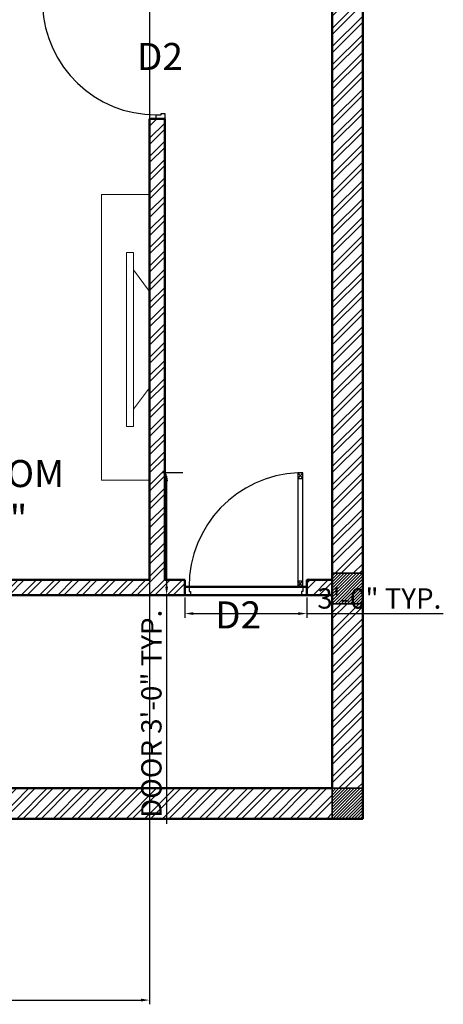
# Model space of a CAD drawing. Units: millimetres. Extents: x 20768 to 23556, y 50760 to 52704.
# Tile 13 of 36: x 21032 to 21157, y 51775 to 52066. Entities that reach past the tile are written whole.
import ezdxf

# ---------------------------------------------------------------- set-up
doc = ezdxf.new("R2010")
doc.units = ezdxf.units.MM
for name, color, linetype, lineweight in [('A-AREA-IDEN', 40, 'Continuous', 18), ('A-DOOR', 3, 'Continuous', 25), ('A-FURN', 8, 'Continuous', 18), ('A-WALL', 7, 'Continuous', 50), ('A-WALL-PATT', 8, 'Continuous', 13), ('S-ANNO-DIMS', 2, 'Continuous', 18), ('S-COLS', 20, 'Continuous', 35)]:
    doc.layers.add(name, color=color, linetype=linetype, lineweight=lineweight)
doc.styles.get("Standard").update_dxf_attribs({"font": 'arial.ttf'})
doc.dimstyles.new('ISO-25', dxfattribs={"dimtxt": 6, "dimasz": 2.5, "dimexe": 1.25, "dimexo": 0.625, "dimtad": 1, "dimdec": 0, "dimlunit": 3, "dimtxsty": 'Standard', "dimcen": 2.5, "dimadec": 0, "dimazin": 0, "dimtfac": 1, "dimtdec": 0, "dimtmove": 0, "dimatfit": 3, "dimfxl": 1, "dimarcsym": 0})
pattern_1 = [(45, (-81.1113, 0), (-2.69407684, 2.69407684), []), (45, (-79.3152, 0), (-2.69407684, 2.69407684), [])]
pattern_2 = [(45, (-81.11126, 0), (-0.449012806, 0.449012806), [])]

# ---------------------------------------------------------------- blocks, each defined once
blk = doc.blocks.new('Puerta 01')
for p, q in [((-0.7745, -0.0264), (-0.7368, -0.0584)), ((-0.7745, -0.0584), (-0.7368, -0.0264)), ((-0.7368, -0.0584), (-0.7368, -0.0264)), ((-0.028, -0.0584), (-0.0657, -0.0264)), ((-0.028, -0.0264), (-0.0657, -0.0584)), ((-0.0657, -0.0584), (-0.0657, -0.0264))]:
    blk.add_line(p, q)
for points in [[(-0.028, 0), (-0.028, -0.0264), (0.004, -0.0264), (0.004, -0.036), (0.028, -0.036), (0.028, 0)], [(-0.028, -0.0264), (-0.7745, -0.0264), (-0.7745, -0.0584), (-0.028, -0.0584)], [(0.004, -0.7736), (0.004, -0.764), (0.028, -0.764), (0.028, -0.8), (-0.028, -0.8), (-0.028, -0.7736)]]:
    blk.add_lwpolyline(points, close=True)
blk.add_arc((-0.028, -0.0264), 0.7472, 182.45453, 270)
blk = doc.blocks.new('tv')
for p, q in [((20989.25, 52437.95), (20993.93, 52444.3)), ((20989.25, 52409.51), (20993.93, 52403.15))]:
    blk.add_line(p, q)
for points in [[(20989.25, 52466.51), (21003.46, 52466.51), (21003.46, 52382.21), (20989.25, 52382.21)], [(20993.93, 52449.42), (20996.05, 52449.42), (20996.05, 52398.03), (20993.93, 52398.03)]]:
    blk.add_lwpolyline(points, close=True)
blk = doc.blocks.new('COL-PLAN')
blk.add_line((0, 9), (9, 9))
blk.add_lwpolyline([(9, 9), (0, 9), (0, 0), (9, 0)], close=True)
blk = doc.blocks.new('*D173')
at = {"layer": 'Defpoints', "color": 0, "transparency": 16777216}
for p in [(21080.64, 51932.01), (21075.22, 51895.9), (21080.64, 51895.9)]:
    blk.add_point(p, dxfattribs=at)
at = {"layer": 'S-ANNO-DIMS', "color": 0, "lineweight": -2, "transparency": 16777216}
for p, q in [((21080.01, 51932.01), (21073.97, 51932.01)), ((21075.22, 51929.51), (21075.22, 51898.4)), ((21080.01, 51895.9), (21073.97, 51895.9)), ((21075.22, 51895.9), (21075.22, 51828.4))]:
    blk.add_line(p, q, dxfattribs=at)
at = {"layer": 'S-ANNO-DIMS', "color": 0, "transparency": 16777216}
for points in [[(21074.81, 51929.51), (21075.64, 51929.51), (21075.22, 51932.01)], [(21074.81, 51898.4), (21075.64, 51898.4), (21075.22, 51895.9)]]:
    blk.add_solid(points, dxfattribs=at)
at = {"layer": 'S-ANNO-DIMS', "color": 0, "transparency": 16777216, "insert": (21071.49, 51860.9), "char_height": 6, "attachment_point": 5, "rotation": 90}
blk.add_mtext('DOOR 3\'-0" TYP.', dxfattribs=at)
blk = doc.blocks.new('*D174')
at = {"layer": 'Defpoints', "color": 0, "transparency": 16777216}
for p in [(21080.64, 51895.9), (21116.64, 51895.9), (21116.64, 51890.48)]:
    blk.add_point(p, dxfattribs=at)
at = {"layer": 'S-ANNO-DIMS', "color": 0, "lineweight": -2, "transparency": 16777216}
for p, q in [((21080.64, 51895.27), (21080.64, 51889.23)), ((21116.64, 51895.27), (21116.64, 51889.23)), ((21083.14, 51890.48), (21114.14, 51890.48)), ((21116.64, 51890.48), (21156.96, 51890.48))]:
    blk.add_line(p, q, dxfattribs=at)
at = {"layer": 'S-ANNO-DIMS', "color": 0, "transparency": 16777216}
for points in [[(21083.14, 51890.9), (21083.14, 51890.06), (21080.64, 51890.48)], [(21114.14, 51890.9), (21114.14, 51890.06), (21116.64, 51890.48)]]:
    blk.add_solid(points, dxfattribs=at)
at = {"layer": 'S-ANNO-DIMS', "color": 0, "transparency": 16777216, "insert": (21138.05, 51894.17), "char_height": 6, "attachment_point": 5}
blk.add_mtext('3\'-0" TYP.', dxfattribs=at)
blk = doc.blocks.new('*D207')
at = {"layer": 'Defpoints', "color": 0, "transparency": 16777216}
for p in [(20908.14, 52080.4), (21070.14, 52080.4), (21070.14, 51776.4)]:
    blk.add_point(p, dxfattribs=at)
at = {"layer": 'S-ANNO-DIMS', "color": 0, "lineweight": -2, "transparency": 16777216}
for p, q in [((20908.14, 52079.77), (20908.14, 51775.15)), ((21070.14, 52079.77), (21070.14, 51775.15)), ((20910.64, 51776.4), (21067.64, 51776.4))]:
    blk.add_line(p, q, dxfattribs=at)
at = {"layer": 'S-ANNO-DIMS', "color": 0, "transparency": 16777216}
for points in [[(20910.64, 51776.81), (20910.64, 51775.98), (20908.14, 51776.4)], [(21067.64, 51776.81), (21067.64, 51775.98), (21070.14, 51776.4)]]:
    blk.add_solid(points, dxfattribs=at)
at = {"layer": 'S-ANNO-DIMS', "color": 0, "transparency": 16777216, "insert": (20989.14, 51780.09), "char_height": 6, "attachment_point": 5}
blk.add_mtext('13\'-6"', dxfattribs=at)

msp = doc.modelspace()

# ---------------------------------------------------------------- hatches: boundary and pattern name
at = {"layer": 'A-WALL-PATT'}
h = msp.add_hatch(dxfattribs=at)
h.set_pattern_fill('ANSI32', color=256, scale=0.4)
h.set_pattern_definition(pattern_1)
h.paths.add_polyline_path([(21133.14, 52075.89), (21124.14, 52075.89), (21124.14, 51902.4), (21133.14, 51902.4)])
h = msp.add_hatch(dxfattribs=at)
h.set_pattern_fill('ANSI32', color=256, scale=0.4)
h.set_pattern_definition(pattern_1)
h.paths.add_polyline_path([(21080.64, 51900.4), (21074.64, 51900.4), (21074.64, 52036.5), (21070.14, 52036.5), (21070.14, 51900.4), (21007.64, 51900.4), (21007.64, 51895.9), (21080.64, 51895.9)])
h = msp.add_hatch(dxfattribs=at)
h.set_pattern_fill('ANSI32', color=256, scale=0.4)
h.set_pattern_definition(pattern_1)
h.paths.add_polyline_path([(21124.14, 51900.4), (21116.64, 51900.4), (21116.64, 51895.9), (21124.14, 51895.9)])
h = msp.add_hatch(dxfattribs=at)
h.set_pattern_fill('ANSI31', color=256, scale=0.2)
h.set_pattern_definition(pattern_2)
h.paths.add_polyline_path([(21133.14, 51902.4), (21124.14, 51902.4), (21124.14, 51893.4), (21133.14, 51893.4)])
h = msp.add_hatch(dxfattribs=at)
h.set_pattern_fill('ANSI32', color=256, scale=0.4)
h.set_pattern_definition(pattern_1)
h.paths.add_polyline_path([(21133.14, 51893.4), (21124.14, 51893.4), (21124.14, 51838.9), (21133.14, 51838.9)])
h = msp.add_hatch(dxfattribs=at)
h.set_pattern_fill('ANSI32', color=256, scale=0.4)
h.set_pattern_definition(pattern_1)
h.paths.add_polyline_path([(21124.14, 51838.9), (20962.14, 51838.9), (20962.14, 51836.13), (20962.14, 51836.13), (20962.14, 51834.4), (20962.14, 51829.9), (21124.14, 51829.9)])
h = msp.add_hatch(dxfattribs=at)
h.set_pattern_fill('ANSI31', color=256, scale=0.2)
h.set_pattern_definition(pattern_2)
h.paths.add_polyline_path([(21133.14, 51838.9), (21124.14, 51838.9), (21124.14, 51829.9), (21133.14, 51829.9)])

# ---------------------------------------------------------------- linework, layer by layer
at = {"layer": 'A-WALL'}
for p, q in [((21133.14, 52522.9), (21133.14, 51829.9)), ((21124.14, 52513.9), (21124.14, 51838.9)), ((21070.14, 52036.5), (21070.14, 51900.4)), ((21070.14, 52036.5), (21074.64, 52036.5)), ((21074.64, 52036.5), (21074.64, 51900.4)), ((20908.14, 51900.4), (21070.14, 51900.4)), ((21074.64, 51900.4), (21080.64, 51900.4)), ((21080.64, 51900.4), (21080.64, 51895.9)), ((21116.64, 51900.4), (21116.64, 51895.9)), ((21116.64, 51900.4), (21124.14, 51900.4)), ((21080.64, 51898.42), (21116.64, 51898.42)), ((20908.14, 51895.9), (21080.64, 51895.9)), ((21080.64, 51895.9), (21116.64, 51895.9)), ((21116.64, 51895.9), (21124.14, 51895.9)), ((20962.14, 51838.9), (21124.14, 51838.9)), ((20962.14, 51829.9), (21133.14, 51829.9))]:
    msp.add_line(p, q, dxfattribs=at)
at = {"layer": 'S-COLS'}
msp.add_lwpolyline([(21133.14, 51829.9), (21124.14, 51829.9), (21124.14, 51838.9), (21133.14, 51838.9)], close=True, dxfattribs=at)

# ---------------------------------------------------------------- block references
at = {"layer": 'A-DOOR', "xscale": 45.00000000000063, "yscale": 45.00000000000063, "zscale": 45.00000000000063}
msp.add_blockref('Puerta 01', (21073.38, 52072.5), dxfattribs=at)
at = {"layer": 'A-DOOR', "xscale": 45.00000000000063, "yscale": 45.00000000000063, "zscale": 45.00000000000063, "rotation": 270.0000000000007}
msp.add_blockref('Puerta 01', (21116.64, 51897.16), dxfattribs=at)
at = {"layer": 'A-FURN', "xscale": -1}
msp.add_blockref('tv', (42059.39, -452.38), dxfattribs=at)
at = {"layer": 'S-COLS'}
msp.add_blockref('COL-PLAN', (21124.14, 51893.4), dxfattribs=at)

# ---------------------------------------------------------------- texts
at = {"layer": 'A-AREA-IDEN', "char_height": 8, "attachment_point": 1}
for s, width, insert in [(' D2', 27.5349, (21064.02, 52058.91)), ('LIVING ROOM\\P    15\'X13\'6"', 94.7826, (20976.48, 51935.81)), (' D2', 27.5349, (21087.11, 51894.08))]:
    msp.add_mtext_dynamic_manual_height_columns(s, width=width, gutter_width=12.5, heights=[0], dxfattribs=dict(at, insert=insert))

# ---------------------------------------------------------------- dimensions: what is measured, and where the dimension line sits
at = {"layer": 'S-ANNO-DIMS'}
dim = msp.add_linear_dim(base=(21070.14, 51776.4), p1=(20908.14, 52080.4), p2=(21070.14, 52080.4), dimstyle='ISO-25', override={"dimdec": 1, "dimlfac": 1, "dimrnd": 0, "dimzin": 1, "dimdsep": 46, "dimlunit": 4, "dimfrac": 2}, dxfattribs=at)
dim.commit()
dim.dimension.update_dxf_attribs({"geometry": '*D207', "text_midpoint": (20989.14, 51780.09)})
for base, p1, p2, angle, text, picture, middle in [((21075.22, 51895.9), (21080.64, 51932.01), (21080.64, 51895.9), 270, 'DOOR <> TYP.', '*D173', (21071.49, 51860.9)), ((21116.64, 51890.48), (21080.64, 51895.9), (21116.64, 51895.9), 0, '<> TYP.', '*D174', (21138.05, 51894.17))]:
    dim = msp.add_linear_dim(base=base, p1=p1, p2=p2, angle=angle, text=text, dimstyle='ISO-25', override={"dimdec": 1, "dimrnd": 0, "dimzin": 1, "dimlunit": 4, "dimfrac": 2}, dxfattribs=at)
    dim.commit()
    dim.dimension.update_dxf_attribs({"geometry": picture, "text_midpoint": middle})

doc.saveas('drawing.dxf')
